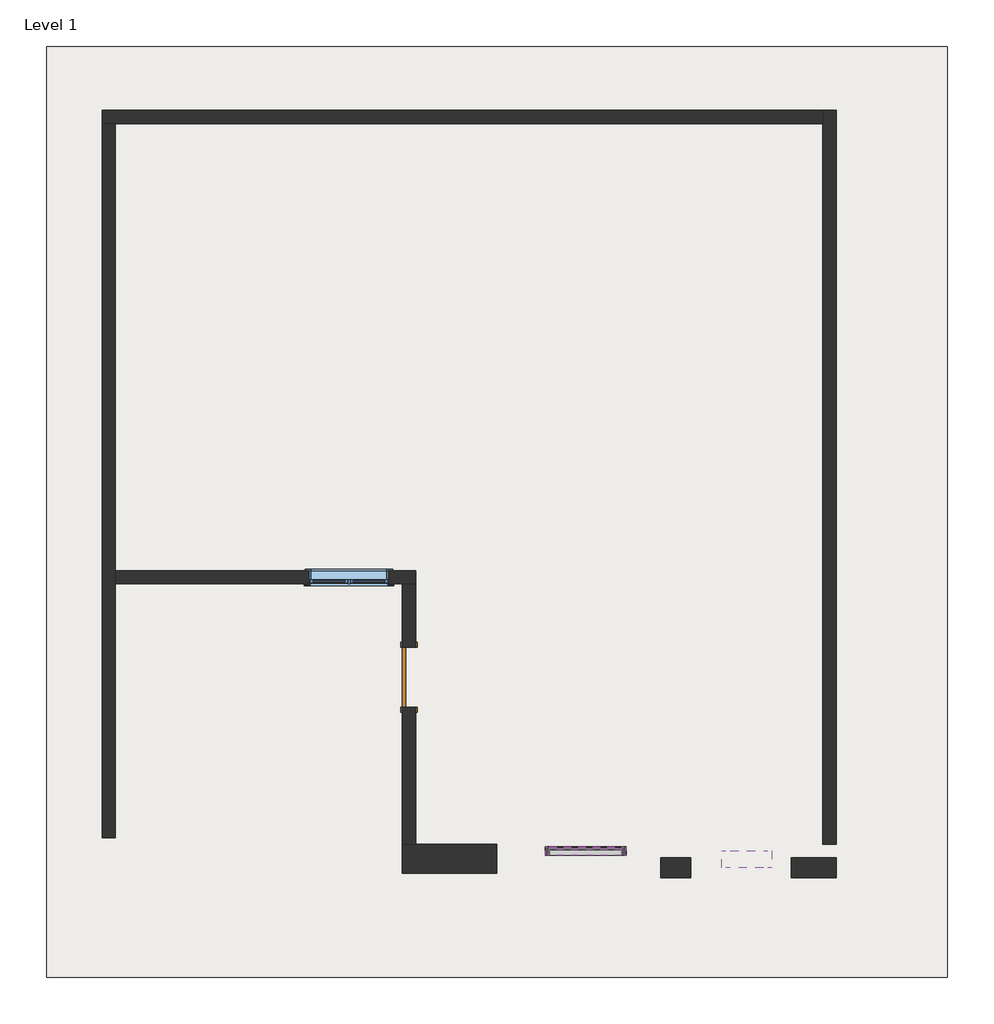
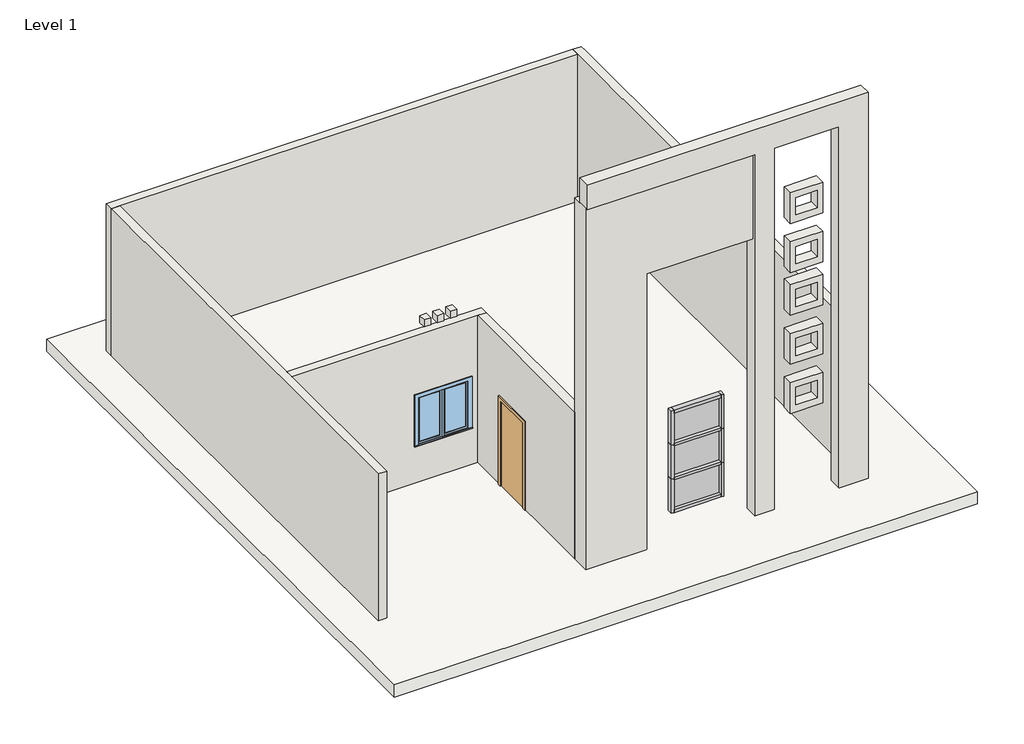
# One storey: 10 members, 7 walls, 3 plates, 1 door, 1 slab, 1 window.
"""IFC4 building model written with IfcOpenShell, lengths in millimetres."""

from ifc_helpers import new_model, si_unit, frame, origin, place, context, project, spatial, polyline, outline, extrude, faceted_brep, transform, mapped, element, save
from components import door_54dd4da4, member_88401a07, member_a8c92c1b, member_62723634, system_panel_glazed_d90ea448, system_panel_glazed_4864a337, walls_1_walls_1_01443282, walls_5_walls_5_6bae5a5a, window_0862ab64

model = new_model("IFC4")

# Units and contexts
model_context = context("Model", 3, world=origin())
ifc_project = project(units=[si_unit("LENGTHUNIT", "METRE", prefix="MILLI")], contexts=[model_context])

# Site, building, storey
site = spatial("IfcSite", under=ifc_project)
building = spatial("IfcBuilding", under=site)
storey = spatial("IfcBuildingStorey", under=building, Name="Level 1", Elevation=0.0)

# Door
placement = place(None, origin())
door_shape = door_54dd4da4(model_context)
element("IfcDoor", 1, ObjectType="Single-Flush : 36\" x 84\"", at=placement, inside=storey, context=model_context, shape_type="MappedRepresentation", body=[
    mapped(door_shape, transform((-6342.5183714, 2519.8900371, 0.0), x_axis=(0.0, 1.0, 0.0), y_axis=(-1.0, 0.0, 0.0), z_axis=(0.0, 0.0, 1.0))),
])

# Members
member_shape = member_88401a07(model_context)
element("IfcMember", 2, ObjectType="Rectangular Mullion : 2.5\" x 5\" rectangular", at=placement, inside=storey, context=model_context, shape_type="MappedRepresentation", body=[
    mapped(member_shape, transform((-3100.8433714, -121.7099629, 2165.1967769), x_axis=(0.0, 0.0, 1.0), y_axis=(0.0, -1.0, 0.0), z_axis=(1.0, 0.0, 0.0))),
])
element("IfcMember", 3, ObjectType="Rectangular Mullion : 2.5\" x 5\" rectangular", at=placement, inside=storey, context=model_context, shape_type="MappedRepresentation", body=[
    mapped(member_shape, transform((-3100.8433714, -121.7099629, 1319.3426601), x_axis=(0.0, 0.0, 1.0), y_axis=(0.0, -1.0, 0.0), z_axis=(1.0, 0.0, 0.0))),
])
member_2_shape = member_a8c92c1b(model_context)
element("IfcMember", 4, ObjectType="Rectangular Mullion : 2.5\" x 5\" rectangular", at=placement, inside=storey, context=model_context, shape_type="MappedRepresentation", body=[
    mapped(member_2_shape, transform((-3100.8433714, -121.7099629, 3011.0508937), x_axis=(0.0, 0.0, 1.0), y_axis=(0.0, -1.0, 0.0), z_axis=(1.0, 0.0, 0.0))),
])
element("IfcMember", 5, ObjectType="Rectangular Mullion : 2.5\" x 5\" rectangular", at=placement, inside=storey, context=model_context, shape_type="MappedRepresentation", body=[
    mapped(member_2_shape, transform((-4203.6276154, -121.7099629, 473.4885433), x_axis=(0.0, 0.0, -1.0), y_axis=(0.0, -1.0, 0.0), z_axis=(-1.0, 0.0, 0.0))),
])
member_3_shape = member_62723634(model_context)
element("IfcMember", 6, ObjectType="Rectangular Mullion : 2.5\" x 5\" rectangular", at=placement, inside=storey, context=model_context, shape_type="MappedRepresentation", body=[
    mapped(member_3_shape, transform((-4267.1276154, -121.7099629, 1319.3426601), x_axis=(-1.0, 0.0, 0.0), y_axis=(0.0, -1.0, 0.0), z_axis=(0.0, 0.0, 1.0))),
])
element("IfcMember", 7, ObjectType="Rectangular Mullion : 2.5\" x 5\" rectangular", at=placement, inside=storey, context=model_context, shape_type="MappedRepresentation", body=[
    mapped(member_3_shape, transform((-4267.1276154, -121.7099629, 2165.1967769), x_axis=(-1.0, 0.0, 0.0), y_axis=(0.0, -1.0, 0.0), z_axis=(0.0, 0.0, 1.0))),
])
element("IfcMember", 8, ObjectType="Rectangular Mullion : 2.5\" x 5\" rectangular", at=placement, inside=storey, context=model_context, shape_type="MappedRepresentation", body=[
    mapped(member_3_shape, transform((-4267.1276154, -121.7099629, 3011.0508937), x_axis=(-1.0, 0.0, 0.0), y_axis=(0.0, -1.0, 0.0), z_axis=(0.0, 0.0, 1.0))),
])
element("IfcMember", 9, ObjectType="Rectangular Mullion : 2.5\" x 5\" rectangular", at=placement, inside=storey, context=model_context, shape_type="MappedRepresentation", body=[
    mapped(member_3_shape, transform((-3037.3433714, -121.7099629, 1319.3426601), x_axis=(1.0, 0.0, 0.0), y_axis=(0.0, -1.0, 0.0), z_axis=(0.0, 0.0, -1.0))),
])
element("IfcMember", 10, ObjectType="Rectangular Mullion : 2.5\" x 5\" rectangular", at=placement, inside=storey, context=model_context, shape_type="MappedRepresentation", body=[
    mapped(member_3_shape, transform((-3037.3433714, -121.7099629, 2165.1967769), x_axis=(1.0, 0.0, 0.0), y_axis=(0.0, -1.0, 0.0), z_axis=(0.0, 0.0, -1.0))),
])
element("IfcMember", 11, ObjectType="Rectangular Mullion : 2.5\" x 5\" rectangular", at=placement, inside=storey, context=model_context, shape_type="MappedRepresentation", body=[
    mapped(member_3_shape, transform((-3037.3433714, -121.7099629, 473.4885433), x_axis=(1.0, 0.0, 0.0), y_axis=(0.0, -1.0, 0.0), z_axis=(0.0, 0.0, -1.0))),
])

# Plates
system_panel_glazed_shape = system_panel_glazed_d90ea448(model_context)
element("IfcPlate", 12, ObjectType="System Panel : Glazed", at=placement, inside=storey, context=model_context, shape_type="MappedRepresentation", body=[
    mapped(system_panel_glazed_shape, transform((-3652.2354934, -121.7099629, 536.9885433), x_axis=(1.0, 0.0, 0.0), y_axis=(0.0, 1.0, 0.0), z_axis=(0.0, 0.0, 1.0))),
])
element("IfcPlate", 13, ObjectType="System Panel : Glazed", at=placement, inside=storey, context=model_context, shape_type="MappedRepresentation", body=[
    mapped(system_panel_glazed_shape, transform((-3652.2354934, -121.7099629, 2196.9467769), x_axis=(1.0, 0.0, 0.0), y_axis=(0.0, 1.0, 0.0), z_axis=(0.0, 0.0, 1.0))),
])
system_panel_glazed_2_shape = system_panel_glazed_4864a337(model_context)
element("IfcPlate", 14, ObjectType="System Panel : Glazed", at=placement, inside=storey, context=model_context, shape_type="MappedRepresentation", body=[
    mapped(system_panel_glazed_2_shape, transform((-3652.2354934, -121.7099629, 1351.0926601), x_axis=(1.0, 0.0, 0.0), y_axis=(0.0, 1.0, 0.0), z_axis=(0.0, 0.0, 1.0))),
])

# Slab
element("IfcSlab", 15, ObjectType="Generic - 12\"", at=placement, inside=storey, context=model_context, shape_type="SweptSolid", body=[
    extrude(outline(polyline([(1855.5059369, 12125.2310952), (1855.5059369, -2047.9689048), (-11860.4940631, -2047.9689048), (-11860.4940631, 12125.2310952), (1855.5059369, 12125.2310952)])), frame((0.0, 0.0, -304.8), z_axis=(0.0, 0.0, 1.0), x_axis=(1.0, 0.0, 0.0)), (0.0, 0.0, 1.0), 304.8),
])

# Walls
element("IfcWall", 16, ObjectType="Generic - 8\"", at=placement, inside=storey, context=model_context, shape_type="Brep", body=[
    faceted_brep([(-11016.1183714, 10952.6900371, 0.0), (-10812.9183714, 10952.6900371, 0.0), (-43.3183714, 10952.6900371, 0.0), (-43.3183714, 10952.6900371, 3657.6), (-10812.9183714, 10952.6900371, 3657.6), (-11016.1183714, 10952.6900371, 3657.6), (-11016.1183714, 11155.8900371, 0.0), (-11016.1183714, 11155.8900371, 3657.6), (-43.3183714, 11155.8900371, 3657.6), (-43.3183714, 11155.8900371, 0.0)], [[[0, 1, 2, 3, 4, 5]], [[6, 7, 8, 9]], [[2, 1, 0, 6, 9]], [[0, 5, 7, 6]], [[3, 2, 9, 8]], [[5, 4, 3, 8, 7]]]),
])
element("IfcWall", 17, ObjectType="Generic - 8\"", at=placement, inside=storey, context=model_context, shape_type="Brep", body=[
    faceted_brep([(-10812.9183714, 81.4900371, 0.0), (-10812.9183714, 3942.2900371, 0.0), (-10812.9183714, 4145.4900371, 0.0), (-10812.9183714, 10952.6900371, 0.0), (-10812.9183714, 10952.6900371, 3657.6), (-10812.9183714, 4145.4900371, 3657.6), (-10812.9183714, 3942.2900371, 3657.6), (-10812.9183714, 81.4900371, 3657.6), (-11016.1183714, 81.4900371, 0.0), (-11016.1183714, 81.4900371, 3657.6), (-11016.1183714, 10952.6900371, 3657.6), (-11016.1183714, 10952.6900371, 0.0)], [[[0, 1, 2, 3, 4, 5, 6, 7]], [[8, 9, 10, 11]], [[3, 2, 1, 0, 8, 11]], [[0, 7, 9, 8]], [[4, 3, 11, 10]], [[7, 6, 5, 4, 10, 9]]]),
])
element("IfcWall", 18, ObjectType="Generic - 8\"", at=placement, inside=storey, context=model_context, shape_type="Brep", body=[
    faceted_brep([(-43.3183714, 11155.8900371, 0.0), (-43.3183714, 10952.6900371, 0.0), (-43.3183714, -20.1099629, 0.0), (-43.3183714, -20.1099629, 3657.6), (-43.3183714, 10952.6900371, 3657.6), (-43.3183714, 11155.8900371, 3657.6), (159.8816286, 11155.8900371, 0.0), (159.8816286, 11155.8900371, 3657.6), (159.8816286, 10952.6900371, 3657.6), (159.8816286, -20.1099629, 3657.6), (159.8816286, -20.1099629, 0.0)], [[[0, 1, 2, 3, 4, 5]], [[6, 7, 8, 9, 10]], [[2, 1, 0, 6, 10]], [[0, 5, 7, 6]], [[5, 4, 3, 9, 8, 7]], [[3, 2, 10, 9]]]),
])
element("IfcWall", 19, ObjectType="Generic - 8\"", at=placement, inside=storey, context=model_context, shape_type="Brep", body=[
    faceted_brep([(-10812.9183714, 3942.2900371, 0.0), (-6444.1183714, 3942.2900371, 0.0), (-6240.9183714, 3942.2900371, 0.0), (-6240.9183714, 3942.2900371, 3657.6), (-6444.1183714, 3942.2900371, 3657.6), (-10812.9183714, 3942.2900371, 3657.6), (-7866.5183714, 3942.2900371, 2133.6), (-6647.3183714, 3942.2900371, 2133.6), (-6647.3183714, 3942.2900371, 914.4), (-7866.5183714, 3942.2900371, 914.4), (-10812.9183714, 4145.4900371, 0.0), (-10812.9183714, 4145.4900371, 3657.6), (-6240.9183714, 4145.4900371, 3657.6), (-6240.9183714, 4145.4900371, 0.0), (-7866.5183714, 4145.4900371, 2133.6), (-7866.5183714, 4145.4900371, 914.4), (-6647.3183714, 4145.4900371, 914.4), (-6647.3183714, 4145.4900371, 2133.6)], [[[0, 1, 2, 3, 4, 5], [6, 7, 8, 9]], [[10, 11, 12, 13], [14, 15, 16, 17]], [[2, 1, 0, 10, 13]], [[0, 5, 11, 10]], [[3, 2, 13, 12]], [[5, 4, 3, 12, 11]], [[15, 14, 6, 9]], [[16, 15, 9, 8]], [[17, 16, 8, 7]], [[14, 17, 7, 6]]]),
])
element("IfcWall", 20, ObjectType="Generic - 8\"", at=placement, inside=storey, context=model_context, shape_type="Brep", body=[
    faceted_brep([(-6444.1183714, 3942.2900371, 0.0), (-6444.1183714, 2977.0900371, 0.0), (-6444.1183714, 2977.0900371, 2133.6), (-6444.1183714, 2062.6900371, 2133.6), (-6444.1183714, 2062.6900371, 0.0), (-6444.1183714, -20.1099629, 0.0), (-6444.1183714, -20.1099629, 3657.6), (-6444.1183714, 1199.0900371, 3657.6), (-6444.1183714, 3942.2900371, 3657.6), (-6240.9183714, 2977.0900371, 2133.6), (-6240.9183714, 2977.0900371, 0.0), (-6240.9183714, 3942.2900371, 0.0), (-6240.9183714, 3942.2900371, 3657.6), (-6240.9183714, 1199.0900371, 3657.6), (-6240.9183714, -20.1099629, 3657.6), (-6240.9183714, -20.1099629, 0.0), (-6240.9183714, 2062.6900371, 0.0), (-6240.9183714, 2062.6900371, 2133.6)], [[[0, 1, 2, 3, 4, 5, 6, 7, 8]], [[9, 10, 11, 12, 13, 14, 15, 16, 17]], [[16, 15, 5, 4]], [[11, 10, 1, 0]], [[0, 8, 12, 11]], [[8, 7, 6, 14, 13, 12]], [[6, 5, 15, 14]], [[2, 1, 10, 9]], [[3, 2, 9, 17]], [[4, 3, 17, 16]]]),
])
walls_1_walls_1_shape = walls_1_walls_1_01443282(model_context)
element("IfcWall", 21, ObjectType="Walls 1 : Walls 1", at=placement, inside=storey, context=model_context, shape_type="MappedRepresentation", body=[
    mapped(walls_1_walls_1_shape, transform((0.0, 0.0, 0.0), x_axis=(1.0, 0.0, 0.0), y_axis=(0.0, 1.0, 0.0), z_axis=(0.0, 0.0, 1.0))),
])
walls_5_walls_5_shape = walls_5_walls_5_6bae5a5a(model_context)
element("IfcWall", 22, ObjectType="Walls 5 : Walls 5", at=placement, inside=storey, context=model_context, shape_type="MappedRepresentation", body=[
    mapped(walls_5_walls_5_shape, transform((0.0, 0.0, 0.0), x_axis=(1.0, 0.0, 0.0), y_axis=(0.0, 1.0, 0.0), z_axis=(0.0, 0.0, 1.0))),
])

# Window
window_shape = window_0862ab64(model_context)
element("IfcWindow", 23, ObjectType="Casement Dbl with Trim.0001 : 48\" x 48\"", at=placement, inside=storey, context=model_context, shape_type="MappedRepresentation", body=[
    mapped(window_shape, transform((-7256.9183714, 4062.9400371, 0.0), x_axis=(-1.0, 0.0, 0.0), y_axis=(0.0, -1.0, 0.0), z_axis=(0.0, 0.0, 1.0))),
])

save(model, "model.ifc")

# Revit data of these elements
# Type "Single-Flush : 36\" x 84\""
#   Type Mark = "1"
#   Construction Type Id = "MDOOR"
#   Assembly Code = "C1020"
#   Analytic Construction = "Metal"
#   Thickness = 0' - 2"
#   Heat Transfer Coefficient (U) = 0.651978 BTU/(h·ft²·°F)
#   Height = 7' - 0"
#   Trim Projection Ext = 0' - 1"
#   Trim Projection Int = 0' - 1"
#   Trim Width = 0' - 3"
#   Width = 3' - 0"
#   Define Thermal Properties by = 1
#   Door Material = Door - Panel
#   Frame Material = Door - Frame
#   Visual Light Transmittance = 0
#   Solar Heat Gain Coefficient = 0
#   Function = (empty or 0)
#   Wall Closure = (empty or 0)
# Type "Rectangular Mullion : 2.5\" x 5\" rectangular"
#   built-in parameter 1007304 = 0.416667 (stored number, unit not read)
#   built-in parameter 1007301 = 0.104167 (stored number, unit not read)
#   built-in parameter 1007300 = 0.104167 (stored number, unit not read)
# Type "System Panel : Glazed"
#   Construction Type Id = "GSP4R"
#   Analytic Construction = "1/8 in Pilkington single glazing"
#   Visual Light Transmittance = 0.9
#   Solar Heat Gain Coefficient = 0.86
#   Heat Transfer Coefficient (U) = 1.18115 BTU/(h·ft²·°F)
# Type "Generic - 12\""
#   Assembly Code = "B1010"
#   Function = 0
#   Layers, outside or top first: 1' - 0" no material (function 1)
# Type "Generic - 8\""
#   Assembly Code = "B2010"
#   Layers, outside or top first: 0' - 8" no material (function 1)
# Type "Casement Dbl with Trim.0001 : 48\" x 48\""
#   Type Mark = "10"
#   Construction Type Id = "GSP4R"
#   Assembly Code = "B2020100"
#   Analytic Construction = "1/8 in Pilkington single glazing"
#   Visual Light Transmittance = 0.9
#   Solar Heat Gain Coefficient = 0.78
#   Heat Transfer Coefficient (U) = 0.6496 BTU/(h·ft²·°F)
#   Height = 4' - 0"
#   Default Sill Height = 3' - 0"
#   Trim Projection - Ext. = 0' - 0 1/2"
#   Trim Projection - Int. = 0' - 0 3/4"
#   Trim Width - Exterior = 0' - 3 1/2"
#   Trim Width - Interior = 0' - 3 1/2"
#   Width = 4' - 0"
#   Window Inset = 0' - 0 3/4"
#   Define Thermal Properties by = 1
#   Glass Pane Material = Glass
#   Sash Material = Sash
#   Trim Exterior Material = Trim
#   Trim Interior Material = Trim
#   Wall Closure = (empty or 0)
# Element 1 (IfcDoor, "Single-Flush : 36\" x 84\"")
#   Phase Created = New Construction
#   Materials on its faces: "Door - Frame", "Door - Panel"
# Elements 2, 3, 4, 5, 6, 7, 8, 9, 10, 11 (IfcMember, "Rectangular Mullion : 2.5\" x 5\" rectangular")
#   Phase Created = New Construction
#   Materials on its faces: "Aluminum"
# Elements 12, 13, 14 (IfcPlate, "System Panel : Glazed")
#   Phase Created = New Construction
#   Materials on its faces: "Glass"
# Element 15 (IfcSlab, "Generic - 12\"")
#   Height Offset From Level = 0' - 0"
#   Phase Created = New Construction
#   Materials on its faces: "Default Floor"
# Elements 16, 17, 18, 19, 20 (IfcWall, "Generic - 8\"")
#   Top Offset = 0' - 0"
#   Base Offset = 0' - 0"
#   Unconnected Height = 12' - 0"
#   wall height = 12' - 0"
#   Phase Created = New Construction
#   Base Constraint = Level 1
#   Materials on its faces: "Default Wall"
# Element 21 (IfcWall, "Walls 1 : Walls 1")
#   Phase Created = New Construction
#   Materials on its faces: "Default Wall"
# Element 22 (IfcWall, "Walls 5 : Walls 5")
#   Phase Created = New Construction
#   Materials on its faces: "Default Wall"
# Element 23 (IfcWindow, "Casement Dbl with Trim.0001 : 48\" x 48\"")
#   Mark = "2"
#   Phase Created = New Construction
#   Materials on its faces: "Sash", "Trim", "Glass"
# Materials
#   "Door - Panel": class "Wood", colour RGB 210 159 95, transparency 0
#   "Door - Frame": colour RGB 118 70 51, transparency 0
#   "Glass": class "Glass", colour RGB 0 128 192, transparency 0.75, Description = "Soda Lime Glass", Cost = 0
#   "Sash": class "Wood", colour RGB 224 178 126, transparency 0
#   "Trim": class "Wood", colour RGB 224 178 126, transparency 0
#   "Aluminum": class "Metal", colour RGB 247 247 247, transparency 0, Description = "Aluminum 6061", Cost = 0
#   "Default Floor": colour RGB 128 128 128, transparency 0
#   "Default Wall": colour RGB 128 128 128, transparency 0
